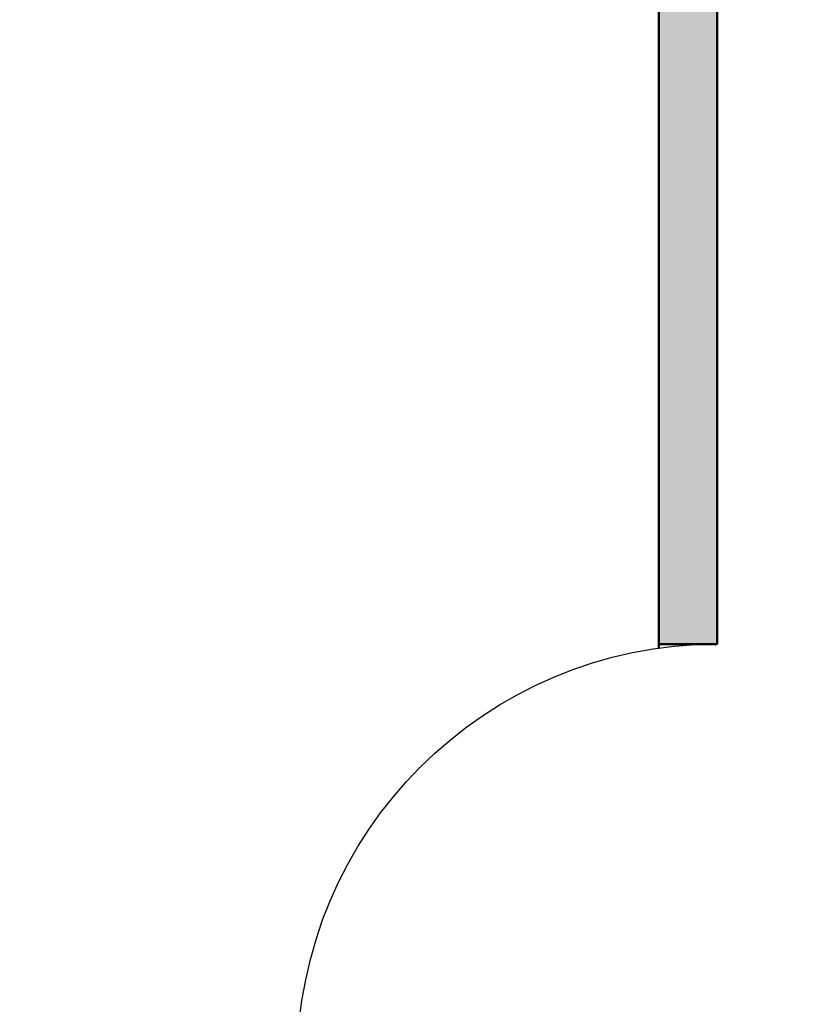
# Model space of a CAD drawing. Units: inches. Extents: x -7 to 1228, y -146 to 1091.
# Tile 31 of 88: x 747 to 815, y 362 to 446. Entities that reach past the tile are written whole.
import ezdxf

# ---------------------------------------------------------------- set-up
doc = ezdxf.new("R2010")
doc.units = ezdxf.units.IN
for name, color, linetype, lineweight in [('A-DOOR', 4, 'Continuous', 25), ('A-WALL', 7, 'Continuous', 50), ('A-WALL-PATT', 251, 'Continuous', 13)]:
    doc.layers.add(name, color=color, linetype=linetype, lineweight=lineweight)

# ---------------------------------------------------------------- blocks, each defined once
blk = doc.blocks.new('DOOR-900')
blk.add_line((36, 0), (36, 36))
blk.add_arc((36, 0), 36, 90, 180)

msp = doc.modelspace()

# ---------------------------------------------------------------- hatches: boundary and pattern name
at = {"layer": 'A-WALL-PATT'}
h = msp.add_hatch(color=256, dxfattribs=at)
h.dxf.hatch_style = 1
h.paths.add_polyline_path([(69, 568), (60, 568), (60, 493), (63.289, 493), (69, 493)])
h.paths.add_polyline_path([(69, 662.405), (60, 662.405), (60, 586), (69, 586)], flags=17)
h.paths.add_polyline_path([(69, 723), (184, 723), (184, 734), (179, 734), (179, 728), (69, 728), (69, 741.623), (60, 741.623), (60, 698.405), (69, 698.405)], flags=17)
h.paths.add_polyline_path([(69, 782), (231, 782), (231, 728), (231, 723), (231, 586), (236, 586), (236, 787), (69, 787), (69, 800.126), (60, 800.126), (60, 765.623), (69, 765.623)])
h.paths.add_polyline_path([(184, 842), (189, 842), (189, 848), (173, 848), (173, 842), (179, 842), (179, 787), (184, 787)])
h.paths.add_polyline_path([(118.22, 69), (69, 69), (69, 60), (118.22, 60)])
h.paths.add_polyline_path([(227, 69), (154.22, 69), (154.22, 60), (227, 60)])
h.paths.add_polyline_path([(236, 60), (232.711, 60), (227, 60), (227, 36), (236, 36)])
h.paths.add_polyline_path([(389, 60), (380, 60), (380, 36), (389, 36)])
h.paths.add_polyline_path([(384, 181), (380, 181), (380, 115), (380, 78), (384, 78)])
h.paths.add_polyline_path([(380, 115), (334.547, 115), (334.547, 109), (380, 109)])
h.paths.add_polyline_path([(274.547, 115), (236, 115), (236, 201), (232.711, 201), (231, 201), (231, 78), (236, 78), (236, 109), (274.547, 109)])
h.paths.add_polyline_path([(69, 123), (60, 123), (60, 78), (69, 78)])
h.paths.add_polyline_path([(69, 201), (60, 201), (60, 159), (69, 159)])
h.paths.add_polyline_path([(143, 219), (69, 219), (69, 213), (143, 213)], flags=17)
h.paths.add_polyline_path([(189, 219), (184, 219), (184, 274), (231, 274), (231, 219), (236, 219), (236, 279), (184, 279), (184, 297), (179, 297), (179, 279), (69, 279), (69, 290.912), (60, 290.912), (60, 262.179), (69, 262.179), (69, 274), (179, 274), (179, 219), (173, 219), (173, 213), (189, 213)])
h.paths.add_polyline_path([(69, 238.179), (60, 238.179), (60, 219), (69, 219)], flags=17)
h.paths.add_polyline_path([(69, 333), (60, 333), (60, 314.912), (69, 314.912), (69, 316.965)])
h.paths.add_polyline_path([(190, 338), (184, 338), (69, 338), (69, 333), (179, 333), (179, 327), (184, 327), (184, 333.021), (190, 333.046)])
h.paths.add_polyline_path([(69, 386.806), (60, 386.806), (60, 351), (69, 351)])
h.paths.add_polyline_path([(69, 475), (60, 475), (60, 422.806), (69, 422.806)])
h.paths.add_polyline_path([(236, 475), (231, 475), (231, 351.238), (236, 351.238)])
h.paths.add_polyline_path([(384, 475), (380, 475), (380, 362), (384, 362)])
h.paths.add_polyline_path([(547, 307), (439, 307), (439, 356), (445, 356), (445, 362), (433, 362), (433, 307), (380, 307), (380, 244), (380, 241), (384, 241), (384, 301), (433, 301), (433, 277), (439, 277), (439, 301), (547, 301)])
h.paths.add_polyline_path([(547, 241), (439, 241), (439, 247), (433, 247), (433, 235), (547, 235)])
h.paths.add_polyline_path([(450, 69), (440.286, 69), (424.889, 69), (389, 69), (389, 60), (450, 60)])
h.paths.add_polyline_path([(547, 69), (486, 69), (486, 60), (547, 60)])
h.paths.add_polyline_path([(556, 148.268), (547, 148.268), (547, 78), (556, 78)])
h.paths.add_polyline_path([(556, 223), (547, 223), (547, 195), (547, 184.268), (556, 184.268)])
h.paths.add_polyline_path([(556, 311.192), (547, 311.192), (547, 273.075), (556, 273.075)])
h.paths.add_polyline_path([(556, 344), (552.711, 344), (547, 344), (547, 335.192), (556, 335.192)])
h.paths.add_polyline_path([(556, 249.075), (547, 249.075), (547, 241), (556, 241)])
h.paths.add_polyline_path([(547, 362), (475, 362), (475, 356), (547, 356)], flags=0)
h.paths.add_polyline_path([(556, 399.621), (547, 399.621), (547, 362), (556, 362)])
h.paths.add_polyline_path([(556, 475), (547, 475), (547, 435.621), (556, 435.621)])
h.paths.add_polyline_path([(547, 493), (389, 493), (389, 487), (547, 487)])
h.paths.add_polyline_path([(380, 493), (278, 493), (278, 487), (380, 487)])
h.paths.add_polyline_path([(227, 493), (69, 493), (69, 487), (227, 487)])
h.paths.add_polyline_path([(643, 122.445), (634, 122.445), (634, 78), (643, 78)])
h.paths.add_polyline_path([(702.5, 69), (692.786, 69), (677.389, 69), (643, 69), (643, 60), (702.5, 60)])
h.paths.add_polyline_path([(798, 69), (738.5, 69), (738.5, 60), (798, 60)])
h.paths.add_polyline_path([(807, 60), (803.711, 60), (798, 60), (798, 36), (807, 36)])
h.paths.add_polyline_path([(807, 109), (846.751, 109), (846.751, 115), (807, 115), (807, 159), (802, 159), (802, 78), (807, 78)])
h.paths.add_polyline_path([(807, 201), (802, 201), (802, 195), (807, 195)])
h.paths.add_polyline_path([(643, 201), (634, 201), (634, 158.445), (643, 158.445)])
h.paths.add_polyline_path([(756, 225), (751, 225), (751, 219), (643, 219), (643, 213), (756, 213)])
h.paths.add_polyline_path([(643, 240.848), (634, 240.848), (634, 219), (643, 219)])
h.paths.add_polyline_path([(643, 274), (643, 288.629), (634, 288.629), (634, 264.848), (643, 264.848)])
h.paths.add_polyline_path([(802, 279), (756, 279), (756, 297), (751, 297), (751, 279), (643, 279), (643, 274), (751, 274), (751, 255), (756, 255), (756, 274), (802, 274)])
h.paths.add_polyline_path([(807, 333), (803.711, 333), (802, 333), (802, 279), (802, 274), (802, 219), (807, 219)])
h.paths.add_polyline_path([(956, 182), (951, 182), (951, 115), (906.751, 115), (906.751, 109), (951, 109), (951, 78), (956, 78)])
h.paths.add_polyline_path([(960, 60), (951, 60), (951, 36), (960, 36)])
h.paths.add_polyline_path([(1021, 69), (1005.781, 69), (960, 69), (960, 60), (1021, 60)])
h.paths.add_polyline_path([(956, 224), (951, 224), (951, 218), (956, 218)])
h.paths.add_polyline_path([(956, 302), (1004, 302), (1004, 278), (1010, 278), (1010, 302), (1118, 302), (1118, 290.809), (1127, 290.809), (1127, 326.968), (1118, 326.968), (1118, 320.966), (1118, 307), (1010, 307), (1010, 356), (1016, 356), (1016, 362), (1004, 362), (1004, 307), (951, 307), (951, 244), (951, 242), (954.289, 242), (956, 242)])
h.paths.add_polyline_path([(643, 333), (634, 333), (634, 312.629), (643, 312.629), (643, 316.965)])
h.paths.add_polyline_path([(756, 338), (643, 338), (643, 333), (751, 333), (751, 327), (756, 327)])
h.paths.add_polyline_path([(643, 388), (634, 388), (634, 351), (643, 351)])
h.paths.add_polyline_path([(807, 357), (802, 357), (802, 351), (807, 351)])
h.paths.add_polyline_path([(807, 475), (802, 475), (802, 393), (807, 393)])
h.paths.add_polyline_path([(643, 475), (634, 475), (634, 424), (643, 424)])
h.paths.add_polyline_path([(798, 493), (643, 493), (643, 487), (798, 487)])
h.paths.add_polyline_path([(634, 493), (556, 493), (556, 487), (634, 487)])
h.paths.add_polyline_path([(813, 493), (807, 493), (807, 487), (813, 487)])
h.paths.add_polyline_path([(951, 493), (849, 493), (849, 487), (951, 487)])
h.paths.add_polyline_path([(956, 484), (951, 484), (951, 374), (956, 374)])
h.paths.add_polyline_path([(1109, 493), (969, 493), (969, 487), (1109, 487)])
h.paths.add_polyline_path([(1127, 484), (1118, 484), (1118, 450.641), (1127, 450.641)])
h.paths.add_polyline_path([(1127, 414.641), (1118, 414.641), (1118, 365), (1127, 365)])
h.paths.add_polyline_path([(1109, 362), (1046, 362), (1046, 356), (1109, 356)], flags=17)
h.paths.add_polyline_path([(1127, 356), (1123.454, 356), (1118, 356), (1118, 350.968), (1127, 350.968)], flags=0)
h.paths.add_polyline_path([(1127, 266.809), (1118, 266.809), (1118, 262.361), (1118, 242), (1127, 242)], flags=17)
h.paths.add_polyline_path([(1118, 242), (1010, 242), (1010, 248), (1004, 248), (1004, 237), (1118, 237)])
h.paths.add_polyline_path([(1127, 224), (1118, 224), (1118, 170), (1127, 170)])
h.paths.add_polyline_path([(1127, 134), (1118, 134), (1118, 78), (1127, 78)])
h.paths.add_polyline_path([(1118, 69), (1057, 69), (1057, 60), (1118, 60)])
h.paths.add_polyline_path([(227, 571.546), (227, 574), (69, 574), (69, 568), (227, 568)])
h.paths.add_polyline_path([(380, 571.546), (380, 574), (278, 574), (278, 568), (380, 568)])
h.paths.add_polyline_path([(242, 574), (236, 574), (236, 568), (242, 568)])
h.paths.add_polyline_path([(547, 571.546), (547, 574), (389, 574), (389, 568), (547, 568)])
h.paths.add_polyline_path([(384, 733), (380, 733), (380, 586), (384, 586)])
h.paths.add_polyline_path([(556, 646), (634, 646), (634, 655), (547, 655), (547, 586), (556, 586)])
h.paths.add_polyline_path([(634, 574), (556, 574), (556, 568), (634, 568)])
h.paths.add_polyline_path([(643, 655), (634, 655), (634, 586), (643, 586)])
h.paths.add_polyline_path([(798, 574), (643, 574), (643, 568), (798, 568)])
h.paths.add_polyline_path([(643, 663.854), (634, 663.854), (634, 655), (643, 655)])
h.paths.add_polyline_path([(556, 676.967), (547, 676.967), (547, 655), (556, 655)])
h.paths.add_polyline_path([(556, 733), (547, 733), (547, 712.967), (556, 712.967)])
h.paths.add_polyline_path([(643, 710), (634, 710), (634, 699.854), (643, 699.854)])
h.paths.add_polyline_path([(807, 668), (802, 668), (802, 586), (807, 586)])
h.paths.add_polyline_path([(951, 574), (849, 574), (849, 568), (951, 568)])
h.paths.add_polyline_path([(956, 691), (951, 691), (951, 577), (956, 577)])
h.paths.add_polyline_path([(1109, 574), (969, 574), (969, 568), (1109, 568)])
h.paths.add_polyline_path([(1127, 643.403), (1118, 643.403), (1118, 577), (1127, 577)])
h.paths.add_polyline_path([(1127, 568), (1123.454, 568), (1118, 568), (1118, 493), (1127, 493)])
h.paths.add_polyline_path([(1127, 733), (1118, 733), (1118, 679.403), (1127, 679.403)])
h.paths.add_polyline_path([(1127, 777.348), (1118, 777.348), (1118, 770.035), (1118, 751), (1127, 751)], flags=17)
h.paths.add_polyline_path([(1118, 751), (1010, 751), (1010, 757), (1004, 757), (1004, 745), (1118, 745)])
h.paths.add_polyline_path([(956, 811), (1004, 811), (1004, 787), (1010, 787), (1010, 811), (1017.874, 811), (1017.874, 811.627, -0.414214), (1018.247, 812), (1031.978, 812, -0.414214), (1032.351, 811.627), (1032.351, 811), (1118, 811), (1118, 801.348), (1127, 801.348), (1127, 834.685), (1118, 834.685), (1118, 830.238), (1118, 817), (1010, 817), (1010, 866), (1016, 866), (1016, 872), (1004, 872), (1004, 817), (956, 817), (956, 866), (951, 866), (951, 751), (954.289, 751), (956, 751)])
h.paths.add_polyline_path([(1118, 872), (1046, 872), (1046, 866), (1118, 866)], flags=17)
h.paths.add_polyline_path([(1127, 924.711), (1118, 924.711), (1118, 884), (1127, 884)])
h.paths.add_polyline_path([(1127, 866), (1123.711, 866), (1118, 866), (1118, 858.685), (1127, 858.685)], flags=17)
h.paths.add_polyline_path([(956, 983), (951, 983), (951, 952), (807, 952), (807, 983), (802, 983), (802, 902), (807, 902), (807, 946), (951, 946), (951, 884), (956, 884)])
h.paths.add_polyline_path([(807, 842), (802, 842), (802, 787), (756, 787), (756, 806), (751, 806), (751, 787), (643, 787), (643, 782), (751, 782), (751, 764), (756, 764), (756, 782), (802, 782), (802, 728), (807, 728)])
h.paths.add_polyline_path([(756, 848), (643, 848), (643, 842), (751, 842), (751, 836), (756, 836)])
h.paths.add_polyline_path([(756, 734), (751, 734), (751, 728), (643, 728), (643, 723), (756, 723)])
h.paths.add_polyline_path([(643, 749.791), (634, 749.791), (634, 728), (637.289, 728), (643, 728)])
h.paths.add_polyline_path([(643, 805.405), (634, 805.405), (634, 773.791), (643, 773.791)])
h.paths.add_polyline_path([(643, 896.663), (634, 896.663), (634, 860), (637.289, 860), (643, 860)])
h.paths.add_polyline_path([(643, 842), (634, 842), (634, 829.405), (643, 829.405)])
h.paths.add_polyline_path([(643, 983), (634, 983), (634, 932.663), (643, 932.663)])
h.paths.add_polyline_path([(1127, 983), (1118, 983), (1118, 960.711), (1127, 960.711)])
h.paths.add_polyline_path([(1118, 1001), (1077.525, 1001), (1077.525, 992), (1118, 992)])
h.paths.add_polyline_path([(1041.525, 1001), (960, 1001), (960, 992), (1041.525, 992)])
h.paths.add_polyline_path([(960, 1025), (951, 1025), (951, 1001), (954.289, 1001), (960, 1001)])
h.paths.add_polyline_path([(807, 1025), (798, 1025), (798, 1001), (807, 1001)])
h.paths.add_polyline_path([(798, 1001), (738.5, 1001), (738.5, 992), (798, 992)])
h.paths.add_polyline_path([(702.5, 1001), (643, 1001), (643, 992), (702.5, 992)])
h.paths.add_polyline_path([(547, 1001), (499.113, 1001), (499.113, 992), (547, 992)])
h.paths.add_polyline_path([(463.113, 1001), (389, 1001), (389, 992), (463.113, 992)])
h.paths.add_polyline_path([(389, 1025), (380, 1025), (380, 1022), (380, 1001), (383.289, 1001), (389, 1001)])
h.paths.add_polyline_path([(236, 1025), (227, 1025), (227, 1001), (236, 1001)])
h.paths.add_polyline_path([(236, 983), (231, 983), (231, 860), (236, 860)])
h.paths.add_polyline_path([(274.547, 952), (236, 952), (236, 946), (274.547, 946)])
h.paths.add_polyline_path([(380, 952), (334.547, 952), (334.547, 946), (380, 946)])
h.paths.add_polyline_path([(384, 983), (380, 983), (380, 884), (383.289, 884), (384, 884)])
h.paths.add_polyline_path([(227, 1001), (155.012, 1001), (155.012, 992), (162.875, 992), (227, 992)])
h.paths.add_polyline_path([(119.012, 1001), (69, 1001), (69, 992), (119.012, 992)])
h.paths.add_polyline_path([(69, 983), (60, 983), (60, 922.987), (69, 922.987)])
h.paths.add_polyline_path([(69, 886.987), (60, 886.987), (60, 860), (63.289, 860), (69, 860)])
h.paths.add_polyline_path([(143, 848), (69, 848), (69, 842), (143, 842)])

# ---------------------------------------------------------------- linework, layer by layer
at = {"layer": 'A-WALL'}
for p, q in [((802, 393), (802, 493)), ((802, 493), (802, 392.651)), ((807, 393), (807, 493)), ((807, 493), (807, 393)), ((807, 393), (802, 393))]:
    msp.add_line(p, q, dxfattribs=at)

# ---------------------------------------------------------------- block references
at = {"layer": 'A-DOOR', "extrusion": (0, 0, -1), "zscale": -1, "rotation": 269.9999999999997}
msp.add_blockref('DOOR-900', (-807, 393), dxfattribs=at)

doc.saveas('drawing.dxf')
